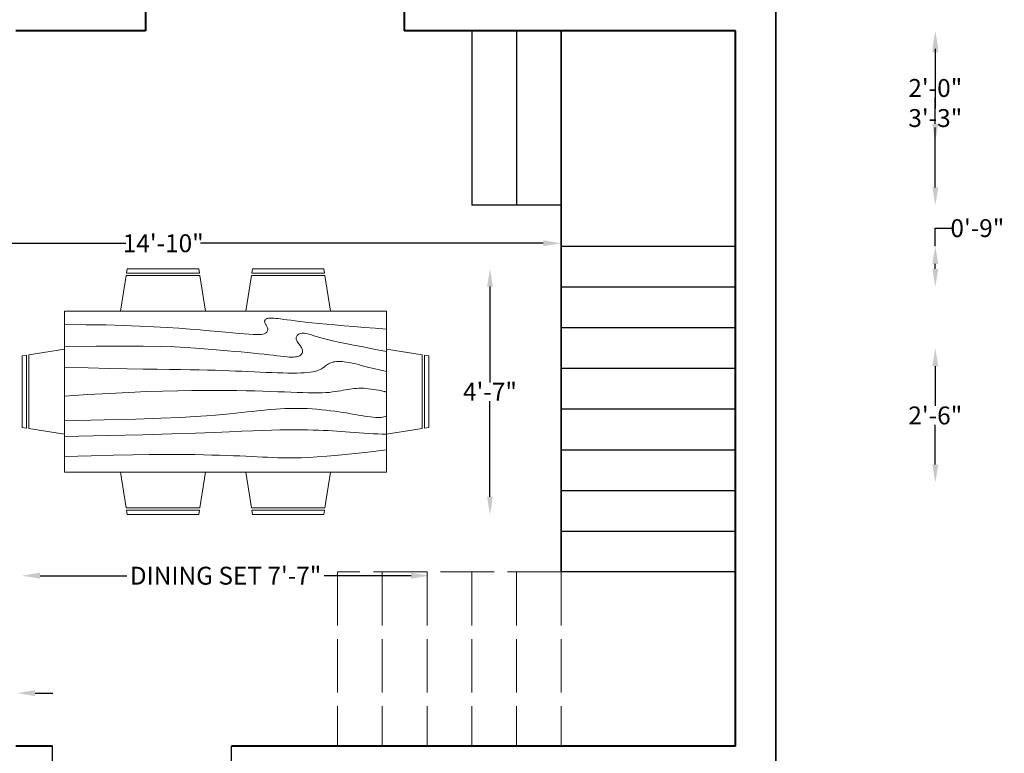
# Model space of a CAD drawing. Units: inches. Extents: x -46 to 447, y -42 to 702.
# Tile 6 of 7: x 227 to 447, y 322 to 487. Entities that reach past the tile are written whole.
import ezdxf

# ---------------------------------------------------------------- set-up
doc = ezdxf.new("R2010")
doc.units = ezdxf.units.IN
doc.header["$PDMODE"] = 3
doc.linetypes.add('ACAD_ISO02W100', pattern=[15, 12, -3])
for name, color, linetype, lineweight in [('A-ANNO-DIMS', 2, 'Continuous', 13), ('A-DOOR', 3, 'Continuous', 25), ('A-FLOR-STRS', 7, 'Continuous', 25), ('A-FLOR-STRS-OVHD', 8, 'ACAD_ISO02W100', 18), ('A-FURN', 8, 'Continuous', 18), ('A-WALL', 7, 'Continuous', 40), ('L-WALL', 7, 'Continuous', 35)]:
    doc.layers.add(name, color=color, linetype=linetype, lineweight=lineweight)
doc.styles.get("Standard").update_dxf_attribs({"font": 'arial.ttf'})
doc.dimstyles.get("Standard").update_dxf_attribs({"dimtxt": 4, "dimasz": 4, "dimexe": 0.18, "dimexo": 0.0625, "dimgap": 0.09, "dimtad": 0, "dimtih": 1, "dimtoh": 1, "dimdec": 0, "dimzin": 0, "dimdsep": 46, "dimlunit": 3, "dimtxsty": 'Standard', "dimcen": 0.09, "dimse1": 1, "dimse2": 1, "dimadec": 0, "dimazin": 0, "dimtfac": 1, "dimtdec": 0, "dimtofl": 0, "dimtmove": 0, "dimatfit": 3, "dimfxl": 1, "dimtolj": 1, "dimtzin": 0, "dimarcsym": 0})

# ---------------------------------------------------------------- blocks, each defined once
blk = doc.blocks.new('*U2')
for p, q in [((0, 0), (0, -6)), ((40, 0), (40, -6))]:
    blk.add_line(p, q)
blk.add_lwpolyline([(0, 0), (0, 40), (1.75, 40), (1.75, 0)], close=True)
blk.add_arc((0, 0), 40, 0, 90)
blk = doc.blocks.new('Dining Set - 36 x 72 in.')
for p, q in [((-22, 27.5), (-22.1562, 26.50042)), ((-5.8416, 26.5), (-22.1534, 26.5)), ((-22, 27.5), (-6, 27.5)), ((-5.8437, 26.49966), (-6, 27.5)), ((6, 27.5), (5.8438, 26.50042)), ((22.1584, 26.5), (5.8466, 26.5)), ((6, 27.5), (22, 27.5)), ((22.1563, 26.49966), (22, 27.5)), ((-22.2343, 26.00059), (-23.4847, 17.99762)), ((-22.2304, 26), (-5.7608, 26)), ((-4.5152, 17.99762), (-5.7655, 25.99926)), ((5.7657, 26.00059), (4.5153, 17.99762)), ((5.7696, 26), (22.2392, 26)), ((23.4848, 17.99762), (22.2345, 25.99926)), ((36, 18), (-36, 18)), ((-36, 18), (-36, -18)), ((36, -18), (36, 18)), ((-44.0006, 8.23428), (-35.9976, 9.48474)), ((44.0006, 8.23428), (35.9976, 9.48474)), ((-45.5, 8), (-44.5004, 8.15617)), ((-45.5, 8), (-45.5, -8)), ((-44.5, -8.15843), (-44.5, 8.15338)), ((-44, 8.23041), (-44, -8.23915)), ((44, 8.23041), (44, -8.23915)), ((44.5, -8.15843), (44.5, 8.15338)), ((45.5, 8), (44.5005, 8.15617)), ((45.5, 8), (45.5, -8)), ((-44.4997, -8.15631), (-45.5, -8)), ((-35.9976, -9.48476), (-43.9993, -8.2345)), ((35.9976, -9.48476), (43.9993, -8.2345)), ((44.4997, -8.15631), (45.5, -8)), ((-36, -18), (36, -18)), ((-22.2343, -26.0006), (-23.4847, -17.99762)), ((-4.5152, -17.99762), (-5.7655, -25.99928)), ((5.7657, -26.0006), (4.5153, -17.99762)), ((23.4848, -17.99762), (22.2345, -25.99928)), ((-22.2304, -26), (-5.7608, -26)), ((5.7696, -26), (22.2392, -26)), ((-22, -27.5), (-22.1562, -26.50044)), ((-5.8416, -26.5), (-22.1534, -26.5)), ((-22, -27.5), (-6, -27.5)), ((-5.8437, -26.49967), (-6, -27.5)), ((6, -27.5), (5.8438, -26.50044)), ((22.1584, -26.5), (5.8466, -26.5)), ((6, -27.5), (22, -27.5)), ((22.1563, -26.49967), (22, -27.5))]:
    blk.add_line(p, q)
for points in [[(-36, 15), (-31.1772, 14.97754), (-26.8079, 14.91406), (-22.8538, 14.81543), (-19.276, 14.6875), (-16.0362, 14.53613), (-13.0957, 14.36718), (-10.4159, 14.18652), (-7.9583, 14), (-5.6904, 13.81315), (-3.6035, 13.63021), (-1.6954, 13.45508), (0.0365, 13.29166), (1.5945, 13.14388), (2.9811, 13.01562), (4.1988, 12.9108), (5.25, 12.83333), (6.1393, 12.78613), (6.8802, 12.76823), (7.4883, 12.77767), (7.9792, 12.8125), (8.3685, 12.87077), (8.6719, 12.95052), (8.9049, 13.0498), (9.0833, 13.16666), (9.2205, 13.29899), (9.3216, 13.44401), (9.3895, 13.59879), (9.4271, 13.76041), (9.4373, 13.92594), (9.4232, 14.09245), (9.3875, 14.257), (9.3333, 14.41666), (9.2638, 14.56917), (9.1836, 14.71484), (9.0975, 14.85465), (9.0104, 14.98958), (8.9272, 15.1206), (8.8529, 15.2487), (8.7922, 15.37483), (8.75, 15.5), (8.7305, 15.62467), (8.7344, 15.74739), (8.7617, 15.86621), (8.8125, 15.97916), (8.8867, 16.08431), (8.9844, 16.17968), (9.1055, 16.26334), (9.25, 16.33333), (9.4189, 16.38802), (9.6172, 16.42708), (9.8506, 16.45052), (10.125, 16.45833), (10.4463, 16.45052), (10.8203, 16.42708), (11.2529, 16.38802), (11.75, 16.33333), (12.3184, 16.26318), (12.9694, 16.17838), (13.7151, 16.07991), (14.5677, 15.96875), (15.5395, 15.84586), (16.6426, 15.71224), (17.8893, 15.56884), (19.2917, 15.41666), (20.859, 15.25667), (22.5879, 15.08984), (24.4721, 14.91715), (26.5052, 14.73958), (28.6809, 14.5581), (30.9929, 14.3737), (33.4347, 14.18733), (36, 14)], [(-36, 10), (-28.9766, 10.14274), (-23.1725, 10.20442), (-18.4241, 10.19775), (-14.5677, 10.13541), (-11.4399, 10.03011), (-8.877, 9.89453), (-6.7154, 9.74137), (-4.7917, 9.58333), (-2.9698, 9.43082), (-1.2246, 9.28515), (0.4415, 9.14534), (2.026, 9.01041), (3.5266, 8.87939), (4.9408, 8.7513), (6.266, 8.62516), (7.5, 8.5), (8.6411, 8.37549), (9.6914, 8.2539), (10.6538, 8.13818), (11.5312, 8.03125), (12.3267, 7.93603), (13.043, 7.85547), (13.6831, 7.79248), (14.25, 7.75), (14.7471, 7.7303), (15.1797, 7.73307), (15.5537, 7.75732), (15.875, 7.80208), (16.1494, 7.86637), (16.3828, 7.94922), (16.5811, 8.04964), (16.75, 8.16666), (16.8944, 8.29915), (17.0143, 8.44531), (17.1089, 8.60319), (17.1771, 8.77083), (17.218, 8.94629), (17.2305, 9.1276), (17.2137, 9.31282), (17.1667, 9.5), (17.0895, 9.6875), (16.987, 9.875), (16.8649, 10.0625), (16.7292, 10.25), (16.5856, 10.4375), (16.4401, 10.625), (16.2985, 10.8125), (16.1667, 11), (16.05, 11.18733), (15.9518, 11.3737), (15.8752, 11.5581), (15.8229, 11.73958), (15.798, 11.91715), (15.8034, 12.08984), (15.842, 12.25667), (15.9167, 12.41666), (16.0295, 12.56836), (16.1784, 12.70833), (16.3605, 12.83268), (16.5729, 12.9375), (16.8127, 13.01888), (17.0768, 13.07291), (17.3625, 13.0957), (17.6667, 13.08333), (17.9894, 13.03312), (18.3418, 12.94726), (18.7382, 12.82918), (19.1927, 12.68229), (19.7195, 12.51001), (20.3327, 12.31575), (21.0465, 12.10294), (21.875, 11.875), (22.8357, 11.63354), (23.959, 11.37304), (25.2786, 11.08618), (26.8282, 10.76562), (28.6414, 10.40405), (30.752, 9.99414), (33.1936, 9.52856), (36, 9)], [(-36, 5.5), (-30.7157, 5.3348), (-26.069, 5.20963), (-21.9946, 5.11767), (-18.4271, 5.05208), (-15.3009, 5.00602), (-12.5508, 4.97265), (-10.1112, 4.94515), (-7.9167, 4.91666), (-5.909, 4.88167), (-4.0586, 4.83984), (-2.3429, 4.79215), (-0.7396, 4.73958), (0.7739, 4.6831), (2.22, 4.6237), (3.6213, 4.56233), (5, 4.5), (6.373, 4.43782), (7.7344, 4.3776), (9.0723, 4.32129), (10.375, 4.27083), (11.6309, 4.22819), (12.8281, 4.19531), (13.9551, 4.17415), (15, 4.16666), (15.954, 4.17448), (16.819, 4.19791), (17.6001, 4.23698), (18.3021, 4.29166), (18.9299, 4.36198), (19.4883, 4.44791), (19.9823, 4.54948), (20.4167, 4.66666), (20.7969, 4.79899), (21.1302, 4.94401), (21.4245, 5.09879), (21.6875, 5.26041), (21.9271, 5.42594), (22.1511, 5.59245), (22.3672, 5.757), (22.5834, 5.91666), (22.8065, 6.06868), (23.0404, 6.21093), (23.2879, 6.34147), (23.5521, 6.45833), (23.8358, 6.55957), (24.142, 6.64323), (24.4735, 6.70735), (24.8334, 6.75), (25.2235, 6.76969), (25.642, 6.76692), (26.0858, 6.74267), (26.5521, 6.69791), (27.0379, 6.63362), (27.5404, 6.55078), (28.0565, 6.45036), (28.5834, 6.33333), (29.1242, 6.19987), (29.7071, 6.04687), (30.3661, 5.87044), (31.1354, 5.66666), (32.0493, 5.43164), (33.142, 5.16146), (34.4475, 4.85221), (36, 4.5)], [(-36, -1), (-30.7915, -0.6591), (-26.0195, -0.38216), (-21.6519, -0.16284), (-17.6563, 0.00521), (-14.0005, 0.12833), (-10.6523, 0.21289), (-7.5796, 0.26522), (-4.75, 0.29166), (-2.134, 0.29793), (0.2878, 0.28711), (2.5317, 0.26163), (4.6146, 0.22396), (6.5529, 0.17651), (8.3633, 0.12174), (10.0623, 0.06209), (11.6667, 0), (13.1899, -0.06201), (14.6341, -0.1211), (15.9982, -0.17432), (17.2813, -0.21875), (18.4823, -0.25147), (19.6003, -0.26953), (20.6343, -0.27002), (21.5834, -0.25), (22.4481, -0.20768), (23.2357, -0.14584), (23.9549, -0.06836), (24.6146, 0.02083), (25.2235, 0.11784), (25.7904, 0.21875), (26.3241, 0.31966), (26.8334, 0.41666), (27.3265, 0.50618), (27.8099, 0.58593), (28.2894, 0.65397), (28.7709, 0.70833), (29.2601, 0.74707), (29.763, 0.76823), (30.2855, 0.76985), (30.8334, 0.75), (31.4088, 0.70784), (31.9994, 0.64713), (32.589, 0.57275), (33.1615, 0.48958), (33.7008, 0.4025), (34.1908, 0.3164), (34.6153, 0.23616), (34.9584, 0.16666), (35.2099, 0.11165), (35.3848, 0.07031), (35.504, 0.04069), (35.5886, 0.02083), (35.6594, 0.00879), (35.7377, 0.0026), (35.8442, 0.00032), (36, 0)], [(-36, -6.5), (-27.1843, -6.31267), (-20.084, -6.1263), (-14.469, -5.9419), (-10.1094, -5.76042), (-6.7752, -5.58285), (-4.2363, -5.41016), (-2.2629, -5.24333), (-0.625, -5.08334), (0.8708, -4.93099), (2.2715, -4.78646), (3.5872, -4.64974), (4.8281, -4.52084), (6.0046, -4.39974), (7.127, -4.28646), (8.2053, -4.18099), (9.25, -4.08334), (10.2705, -3.99382), (11.2734, -3.91407), (12.2647, -3.84603), (13.25, -3.79167), (14.2354, -3.75293), (15.2266, -3.73177), (16.2295, -3.73015), (17.25, -3.75), (18.2912, -3.79248), (19.3451, -3.85547), (20.4009, -3.93604), (21.4479, -4.03125), (22.4754, -4.13819), (23.4727, -4.25391), (24.4289, -4.37549), (25.3334, -4.5), (26.1785, -4.62492), (26.9694, -4.74935), (27.7145, -4.87281), (28.4219, -4.99479), (29.1, -5.11483), (29.7572, -5.23242), (30.4016, -5.34709), (31.0417, -5.45834), (31.6837, -5.56437), (32.3262, -5.65821), (32.9658, -5.73153), (33.599, -5.77604), (34.2224, -5.78345), (34.8327, -5.74545), (35.4264, -5.65373), (36, -5.5)], [(-36, -10), (-26.4022, -9.81299), (-18.4675, -9.62891), (-11.9839, -9.45069), (-6.7396, -9.28125), (-2.5226, -9.12354), (0.8789, -8.98047), (3.6769, -8.85498), (6.0833, -8.75), (8.2767, -8.66765), (10.3021, -8.60677), (12.1712, -8.56543), (13.8958, -8.54167), (15.4876, -8.53353), (16.9583, -8.53907), (18.3197, -8.55632), (19.5834, -8.58334), (20.7616, -8.61841), (21.8685, -8.66081), (22.9188, -8.71004), (23.9271, -8.76563), (24.9081, -8.82707), (25.8763, -8.89388), (26.8465, -8.96558), (27.8334, -9.04167), (28.8474, -9.12118), (29.8828, -9.20117), (30.93, -9.27824), (31.9792, -9.34896), (33.0205, -9.40991), (34.0443, -9.45768), (35.0407, -9.48885), (36, -9.5)], [(-36, -14.5), (-30.0881, -14.33513), (-25.0332, -14.21224), (-20.7312, -14.12647), (-17.0781, -14.07292), (-13.97, -14.04671), (-11.3027, -14.04297), (-8.9724, -14.05681), (-6.875, -14.08334), (-4.9224, -14.11833), (-3.0905, -14.16016), (-1.3709, -14.20785), (0.2448, -14.26042), (1.7647, -14.3169), (3.1973, -14.3763), (4.5507, -14.43767), (5.8333, -14.5), (7.0554, -14.5621), (8.235, -14.62175), (9.3922, -14.67652), (10.5469, -14.72396), (11.7192, -14.76164), (12.929, -14.78711), (14.1965, -14.79794), (15.5417, -14.79167), (16.9933, -14.76424), (18.6152, -14.70508), (20.4804, -14.60197), (22.6615, -14.44271), (25.2312, -14.21509), (28.2624, -13.9069), (31.8277, -13.50594), (36, -13)]]:
    blk.add_lwpolyline(points)
blk = doc.blocks.new('*D61')
at = {"layer": 'A-ANNO-DIMS', "color": 0, "lineweight": -2, "transparency": 16777216}
for p, q in [((174, 436.51), (250.67, 436.51)), ((344, 436.51), (267.33, 436.51))]:
    blk.add_line(p, q, dxfattribs=at)
at = {"layer": 'A-ANNO-DIMS', "color": 0, "transparency": 16777216}
for points in [[(174, 437.18), (174, 435.84), (170, 436.51)], [(344, 437.18), (344, 435.84), (348, 436.51)]]:
    blk.add_solid(points, dxfattribs=at)
at = {"layer": 'Defpoints', "color": 0, "transparency": 16777216}
for p in [(170, 468.57), (348, 468.57), (348, 436.51)]:
    blk.add_point(p, dxfattribs=at)
at = {"layer": 'A-ANNO-DIMS', "color": 0, "transparency": 16777216, "insert": (259, 436.51), "char_height": 4, "attachment_point": 5}
blk.add_mtext('\\A1;14\'-10"', dxfattribs=at)
blk = doc.blocks.new('*D62')
at = {"layer": 'A-ANNO-DIMS', "color": 0, "lineweight": -2, "transparency": 16777216}
for p, q in [((186.57, 480), (186.57, 406.13)), ((186.57, 328), (186.57, 401.87))]:
    blk.add_line(p, q, dxfattribs=at)
at = {"layer": 'A-ANNO-DIMS', "color": 0, "transparency": 16777216}
for points in [[(185.91, 480), (187.24, 480), (186.57, 484)], [(185.91, 328), (187.24, 328), (186.57, 324)]]:
    blk.add_solid(points, dxfattribs=at)
at = {"layer": 'Defpoints', "color": 0, "transparency": 16777216}
for p in [(312.89, 484), (186.57, 324), (312.89, 324)]:
    blk.add_point(p, dxfattribs=at)
at = {"layer": 'A-ANNO-DIMS', "color": 0, "transparency": 16777216, "insert": (186.57, 404), "char_height": 4, "attachment_point": 5}
blk.add_mtext('\\A1;13\'-4"', dxfattribs=at)
blk = doc.blocks.new('*D104')
at = {"layer": 'A-ANNO-DIMS', "color": 0, "lineweight": -2, "transparency": 16777216}
for p, q in [((231.44, 362.16), (250.86, 362.16)), ((314.44, 362.16), (295.01, 362.16))]:
    blk.add_line(p, q, dxfattribs=at)
at = {"layer": 'A-ANNO-DIMS', "color": 0, "transparency": 16777216}
for points in [[(231.44, 362.82), (231.44, 361.49), (227.44, 362.16)], [(314.44, 362.82), (314.44, 361.49), (318.44, 362.16)]]:
    blk.add_solid(points, dxfattribs=at)
at = {"layer": 'Defpoints', "color": 0, "transparency": 16777216}
for p in [(227.44, 375.81), (318.44, 375.81), (318.44, 362.16)]:
    blk.add_point(p, dxfattribs=at)
at = {"layer": 'A-ANNO-DIMS', "color": 0, "transparency": 16777216, "insert": (272.94, 362.16), "char_height": 4, "attachment_point": 5}
blk.add_mtext('\\A1;DINING SET 7\'-7"', dxfattribs=at)
blk = doc.blocks.new('*D105')
at = {"layer": 'A-ANNO-DIMS', "color": 0, "lineweight": -2, "transparency": 16777216}
for p, q in [((332.09, 426.81), (332.09, 405.4)), ((332.09, 379.81), (332.09, 401.22))]:
    blk.add_line(p, q, dxfattribs=at)
at = {"layer": 'A-ANNO-DIMS', "color": 0, "transparency": 16777216}
for points in [[(331.42, 426.81), (332.75, 426.81), (332.09, 430.81)], [(331.42, 379.81), (332.75, 379.81), (332.09, 375.81)]]:
    blk.add_solid(points, dxfattribs=at)
at = {"layer": 'Defpoints', "color": 0, "transparency": 16777216}
for p in [(318.44, 430.81), (332.09, 430.81), (318.44, 375.81)]:
    blk.add_point(p, dxfattribs=at)
at = {"layer": 'A-ANNO-DIMS', "color": 0, "transparency": 16777216, "insert": (332.09, 403.31), "char_height": 4, "attachment_point": 5}
blk.add_mtext('\\A1;4\'-7"', dxfattribs=at)
blk = doc.blocks.new('*D107')
at = {"layer": 'A-ANNO-DIMS', "color": 0, "lineweight": -2, "transparency": 16777216}
for p, q in [((185.68, 335.9), (181.68, 335.9)), ((230.34, 335.9), (234.34, 335.9))]:
    blk.add_line(p, q, dxfattribs=at)
at = {"layer": 'A-ANNO-DIMS', "color": 0, "transparency": 16777216}
for points in [[(185.68, 336.57), (185.68, 335.24), (189.68, 335.9)], [(230.34, 336.57), (230.34, 335.24), (226.34, 335.9)]]:
    blk.add_solid(points, dxfattribs=at)
at = {"layer": 'Defpoints', "color": 0, "transparency": 16777216}
for p in [(226.34, 335.9), (189.68, 326.9), (226.34, 326.9)]:
    blk.add_point(p, dxfattribs=at)
at = {"layer": 'A-ANNO-DIMS', "color": 0, "transparency": 16777216, "insert": (208.01, 335.9), "char_height": 4, "attachment_point": 5}
blk.add_mtext('\\A1;3\'-0 1/2" TYP.', dxfattribs=at)
blk = doc.blocks.new('*D118')
at = {"layer": 'A-ANNO-DIMS', "color": 0, "lineweight": -2, "transparency": 16777216}
for p, q in [((352, -35.7), (362.09, -35.7)), ((383, -35.7), (372.91, -35.7))]:
    blk.add_line(p, q, dxfattribs=at)
at = {"layer": 'A-ANNO-DIMS', "color": 0, "transparency": 16777216}
for points in [[(352, -35.03), (352, -36.37), (348, -35.7)], [(383, -35.03), (383, -36.37), (387, -35.7)]]:
    blk.add_solid(points, dxfattribs=at)
at = {"layer": 'Defpoints', "color": 0, "transparency": 16777216}
for p in [(348, 324), (387, 324), (387, -35.7)]:
    blk.add_point(p, dxfattribs=at)
at = {"layer": 'A-ANNO-DIMS', "color": 0, "transparency": 16777216, "insert": (367.5, -35.7), "char_height": 4, "attachment_point": 5}
blk.add_mtext('\\A1;3\'-3"', dxfattribs=at)
blk = doc.blocks.new('*D119')
at = {"layer": 'A-ANNO-DIMS', "color": 0, "lineweight": -2, "transparency": 16777216}
for p, q in [((238.24, 695.7), (248.83, 695.7)), ((270.24, 695.7), (259.64, 695.7))]:
    blk.add_line(p, q, dxfattribs=at)
at = {"layer": 'A-ANNO-DIMS', "color": 0, "transparency": 16777216}
for points in [[(238.24, 696.37), (238.24, 695.03), (234.24, 695.7)], [(270.24, 696.37), (270.24, 695.03), (274.24, 695.7)]]:
    blk.add_solid(points, dxfattribs=at)
at = {"layer": 'Defpoints', "color": 0, "transparency": 16777216}
for p in [(274.24, 695.7), (234.24, 319), (274.24, 319)]:
    blk.add_point(p, dxfattribs=at)
at = {"layer": 'A-ANNO-DIMS', "color": 0, "transparency": 16777216, "insert": (254.24, 695.7), "char_height": 4, "attachment_point": 5}
blk.add_mtext('\\A1;3\'-4"', dxfattribs=at)
blk = doc.blocks.new('*D126')
at = {"layer": 'A-ANNO-DIMS', "color": 0, "lineweight": -2, "transparency": 16777216}
for p, q in [((431.7, 409), (431.7, 400.13)), ((431.7, 387), (431.7, 395.87))]:
    blk.add_line(p, q, dxfattribs=at)
at = {"layer": 'A-ANNO-DIMS', "color": 0, "transparency": 16777216}
for points in [[(431.03, 409), (432.37, 409), (431.7, 413)], [(431.03, 387), (432.37, 387), (431.7, 383)]]:
    blk.add_solid(points, dxfattribs=at)
at = {"layer": 'Defpoints', "color": 0, "transparency": 16777216}
for p in [(122, 413), (431.7, 413), (122.75, 383)]:
    blk.add_point(p, dxfattribs=at)
at = {"layer": 'A-ANNO-DIMS', "color": 0, "transparency": 16777216, "insert": (431.7, 398), "char_height": 4, "attachment_point": 5}
blk.add_mtext('\\A1;2\'-6"', dxfattribs=at)
blk = doc.blocks.new('*D127')
at = {"layer": 'A-ANNO-DIMS', "color": 0, "lineweight": -2, "transparency": 16777216}
for p, q in [((431.7, 479.23), (431.7, 473.36)), ((431.7, 463.23), (431.7, 469.1))]:
    blk.add_line(p, q, dxfattribs=at)
at = {"layer": 'A-ANNO-DIMS', "color": 0, "transparency": 16777216}
for points in [[(431.03, 479.23), (432.37, 479.23), (431.7, 483.23)], [(431.03, 463.23), (432.37, 463.23), (431.7, 459.23)]]:
    blk.add_solid(points, dxfattribs=at)
at = {"layer": 'Defpoints', "color": 0, "transparency": 16777216}
for p in [(105, 483.23), (431.7, 483.23), (105, 459.23)]:
    blk.add_point(p, dxfattribs=at)
at = {"layer": 'A-ANNO-DIMS', "color": 0, "transparency": 16777216, "insert": (431.7, 471.23), "char_height": 4, "attachment_point": 5}
blk.add_mtext('\\A1;2\'-0"', dxfattribs=at)
blk = doc.blocks.new('*D137')
at = {"layer": 'A-ANNO-DIMS', "color": 0, "lineweight": -2, "transparency": 16777216}
for p, q in [((431.7, 435.89), (431.7, 439.89)), ((431.7, 439.89), (435.7, 439.89)), ((431.7, 430.78), (431.7, 431.89))]:
    blk.add_line(p, q, dxfattribs=at)
at = {"layer": 'A-ANNO-DIMS', "color": 0, "transparency": 16777216}
for points in [[(431.03, 431.89), (432.37, 431.89), (431.7, 435.89)], [(431.03, 430.78), (432.37, 430.78), (431.7, 426.78)]]:
    blk.add_solid(points, dxfattribs=at)
at = {"layer": 'Defpoints', "color": 0, "transparency": 16777216}
for p in [(387, 435.89), (431.7, 435.89), (387, 426.78)]:
    blk.add_point(p, dxfattribs=at)
at = {"layer": 'A-ANNO-DIMS', "color": 0, "transparency": 16777216, "insert": (441.11, 439.89), "char_height": 4, "attachment_point": 5}
blk.add_mtext('\\A1;0\'-9"', dxfattribs=at)
blk = doc.blocks.new('*D148')
at = {"layer": 'A-ANNO-DIMS', "color": 0, "lineweight": -2, "transparency": 16777216}
for p, q in [((227, 695.7), (223, 695.7)), ((238.24, 695.7), (242.24, 695.7))]:
    blk.add_line(p, q, dxfattribs=at)
at = {"layer": 'A-ANNO-DIMS', "color": 0, "transparency": 16777216}
for points in [[(227, 696.37), (227, 695.03), (231, 695.7)], [(238.24, 696.37), (238.24, 695.03), (234.24, 695.7)]]:
    blk.add_solid(points, dxfattribs=at)
at = {"layer": 'Defpoints', "color": 0, "transparency": 16777216}
for p in [(234.24, 695.7), (231, 319), (234.24, 319)]:
    blk.add_point(p, dxfattribs=at)
at = {"layer": 'A-ANNO-DIMS', "color": 0, "transparency": 16777216, "insert": (247.64, 695.7), "char_height": 4, "attachment_point": 5}
blk.add_mtext('\\A1;0\'-3"', dxfattribs=at)
blk = doc.blocks.new('*D149')
at = {"layer": 'A-ANNO-DIMS', "color": 0, "lineweight": -2, "transparency": 16777216}
for p, q in [((332, 695.7), (334, 695.7)), ((338, 695.7), (342, 695.7))]:
    blk.add_line(p, q, dxfattribs=at)
at = {"layer": 'A-ANNO-DIMS', "color": 0, "transparency": 16777216}
for points in [[(332, 696.37), (332, 695.03), (328, 695.7)], [(334, 696.37), (334, 695.03), (338, 695.7)]]:
    blk.add_solid(points, dxfattribs=at)
at = {"layer": 'Defpoints', "color": 0, "transparency": 16777216}
for p in [(338, 695.7), (328, 445), (338, 445)]:
    blk.add_point(p, dxfattribs=at)
at = {"layer": 'A-ANNO-DIMS', "color": 0, "transparency": 16777216, "insert": (348.96, 695.7), "char_height": 4, "attachment_point": 5}
blk.add_mtext('\\A1;0\'-10"', dxfattribs=at)
blk = doc.blocks.new('*D150')
at = {"layer": 'A-ANNO-DIMS', "color": 0, "lineweight": -2, "transparency": 16777216}
for p, q in [((431.7, 480), (431.7, 466.63)), ((431.7, 449), (431.7, 462.37))]:
    blk.add_line(p, q, dxfattribs=at)
at = {"layer": 'A-ANNO-DIMS', "color": 0, "transparency": 16777216}
for points in [[(431.03, 480), (432.37, 480), (431.7, 484)], [(431.03, 449), (432.37, 449), (431.7, 445)]]:
    blk.add_solid(points, dxfattribs=at)
at = {"layer": 'Defpoints', "color": 0, "transparency": 16777216}
for p in [(348, 484), (431.7, 484), (348, 445)]:
    blk.add_point(p, dxfattribs=at)
at = {"layer": 'A-ANNO-DIMS', "color": 0, "transparency": 16777216, "insert": (431.7, 464.5), "char_height": 4, "attachment_point": 5}
blk.add_mtext('\\A1;3\'-3"', dxfattribs=at)

msp = doc.modelspace()

# ---------------------------------------------------------------- linework, layer by layer
at = {"layer": 'A-FLOR-STRS'}
for p, q in [((328, 484), (328, 445)), ((338, 484), (338, 445)), ((348, 363), (348, 484)), ((348, 484), (348, 445)), ((348, 445), (328, 445)), ((348, 445), (348, 363)), ((348, 435.89), (387, 435.89)), ((348, 426.78), (387, 426.78)), ((348, 417.67), (387, 417.67)), ((348, 408.56), (387, 408.56)), ((348, 399.44), (387, 399.44)), ((348, 390.33), (387, 390.33)), ((348, 381.22), (387, 381.22)), ((348, 372.11), (387, 372.11)), ((387, 363), (348, 363))]:
    msp.add_line(p, q, dxfattribs=at)
at = {"layer": 'A-FLOR-STRS-OVHD'}
for p, q in [((298, 363), (298, 324)), ((348, 363), (298, 363)), ((308, 363), (308, 324)), ((318, 363), (318, 324)), ((328, 363), (328, 324)), ((338, 363), (338, 324)), ((348, 363), (348, 324))]:
    msp.add_line(p, q, dxfattribs=at)
at = {"layer": 'A-WALL'}
for p, q in [((255, 489), (255, 484)), ((312.89, 489), (312.89, 484)), ((255, 484), (226, 484)), ((387, 484), (312.89, 484)), ((387, 324), (387, 484)), ((234.24, 324), (226, 324)), ((387, 324), (274.24, 324))]:
    msp.add_line(p, q, dxfattribs=at)
at = {"layer": 'L-WALL'}
msp.add_lwpolyline([(222, 0), (396, 0), (396, 660), (0, 660), (0, 0), (17.93, 0)], dxfattribs=at)

# ---------------------------------------------------------------- block references
at = {"layer": 'A-DOOR', "xscale": -1, "rotation": 180}
msp.add_blockref('*U2', (234.24, 318), dxfattribs=at)
at = {"layer": 'A-FURN'}
msp.add_blockref('Dining Set - 36 x 72 in.', (272.94, 403.31), dxfattribs=at)

# ---------------------------------------------------------------- dimensions: what is measured, and where the dimension line sits
at = {"layer": 'A-ANNO-DIMS'}
for base, p1, p2, override, picture, middle in [((234.24, 695.7), (231, 319), (234.24, 319), {"dimdec": 1, "dimlfac": 1, "dimrnd": 0, "dimzin": 1, "dimdsep": 46, "dimlunit": 4, "dimfrac": 2}, '*D148', (247.64, 695.7)), ((274.24, 695.7), (234.24, 319), (274.24, 319), {"dimdec": 1, "dimlfac": 1, "dimrnd": 0, "dimzin": 1, "dimdsep": 46, "dimlunit": 4, "dimfrac": 2}, '*D119', (254.24, 695.7)), ((338, 695.7), (328, 445), (338, 445), {"dimdec": 1, "dimlfac": 1, "dimrnd": 0, "dimzin": 1, "dimdsep": 46, "dimlunit": 4, "dimfrac": 2}, '*D149', (348.96, 695.7)), ((348, 436.51), (170, 468.57), (348, 468.57), {"dimclrd": 0, "dimclre": 0, "dimclrt": 0}, '*D61', (259, 436.51)), ((387, -35.7), (348, 324), (387, 324), {"dimdec": 1, "dimlfac": 1, "dimrnd": 0, "dimzin": 1, "dimdsep": 46, "dimlunit": 4, "dimfrac": 2}, '*D118', (367.5, -35.7))]:
    dim = msp.add_linear_dim(base=base, p1=p1, p2=p2, dimstyle='Standard', override=override, dxfattribs=at)
    dim.commit()
    dim.dimension.update_dxf_attribs({"geometry": picture, "text_midpoint": middle})
for base, p1, p2, override, picture, middle in [((431.7, 483.23), (105, 459.23), (105, 483.23), {"dimdec": 1, "dimlfac": 1, "dimrnd": 0, "dimzin": 1, "dimdsep": 46, "dimlunit": 4, "dimfrac": 2}, '*D127', (431.7, 471.23)), ((186.57, 324), (312.89, 484), (312.89, 324), {"dimclrd": 0, "dimclre": 0, "dimclrt": 0}, '*D62', (186.57, 404)), ((431.7, 484), (348, 445), (348, 484), {"dimdec": 1, "dimlfac": 1, "dimrnd": 0, "dimzin": 1, "dimdsep": 46, "dimlunit": 4, "dimfrac": 2}, '*D150', (431.7, 464.5)), ((431.7, 435.89), (387, 426.78), (387, 435.89), {"dimdec": 1, "dimlfac": 1, "dimrnd": 0, "dimzin": 1, "dimdsep": 46, "dimlunit": 4, "dimfrac": 2}, '*D137', (441.11, 439.89)), ((332.09, 430.81), (318.44, 375.81), (318.44, 430.81), {"dimdec": 1, "dimlfac": 1, "dimrnd": 0, "dimzin": 1, "dimdsep": 46, "dimlunit": 4, "dimfrac": 2}, '*D105', (332.09, 403.31)), ((431.7, 413), (122.75, 383), (122, 413), {"dimdec": 1, "dimlfac": 1, "dimrnd": 0, "dimzin": 1, "dimdsep": 46, "dimlunit": 4, "dimfrac": 2}, '*D126', (431.7, 398))]:
    dim = msp.add_linear_dim(base=base, p1=p1, p2=p2, angle=90, dimstyle='Standard', override=override, dxfattribs=at)
    dim.commit()
    dim.dimension.update_dxf_attribs({"geometry": picture, "text_midpoint": middle})
for base, p1, p2, text, picture, middle in [((318.44, 362.16), (227.44, 375.81), (318.44, 375.81), 'DINING SET <>', '*D104', (272.94, 362.16)), ((226.34, 335.9), (189.68, 326.9), (226.34, 326.9), '<> TYP.', '*D107', (208.01, 335.9))]:
    dim = msp.add_linear_dim(base=base, p1=p1, p2=p2, text=text, dimstyle='Standard', override={"dimdec": 1, "dimlfac": 1, "dimrnd": 0, "dimzin": 1, "dimdsep": 46, "dimlunit": 4, "dimfrac": 2}, dxfattribs=at)
    dim.commit()
    dim.dimension.update_dxf_attribs({"geometry": picture, "text_midpoint": middle})

doc.saveas('drawing.dxf')
